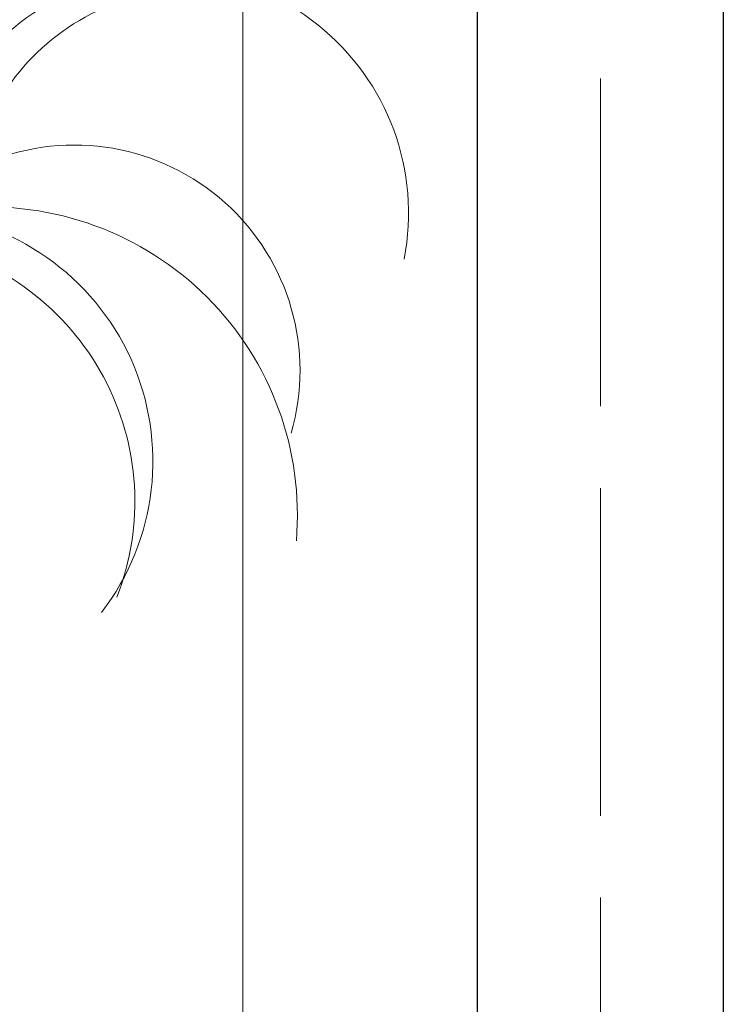
# Model space of a CAD drawing. Units: millimetres. Extents: x 595116 to 630915, y 909473 to 920225.
# Tile 109 of 134: x 629817 to 629843, y 919181 to 919217. Entities that reach past the tile are written whole.
import ezdxf

# ---------------------------------------------------------------- set-up
doc = ezdxf.new("R2010")
doc.units = ezdxf.units.MM
doc.linetypes.add('ACAD_ISO02W100', pattern=[15, 12, -3])
for name, color, linetype, lineweight in [('C-PROP', 7, 'Continuous', 25), ('C-PROP-REF', 240, 'ACAD_ISO02W100', 13), ('L-PLNT', 85, 'Continuous', 13)]:
    doc.layers.add(name, color=color, linetype=linetype, lineweight=lineweight)

# ---------------------------------------------------------------- blocks, each defined once
blk = doc.blocks.new('tree')
for centre, radius, start, end in [((629595.141, 919296.95), 5.184, 352.032, 57.0714), ((629604.232, 919296.737), 3.791, 61.1347, 193.108), ((629569.835, 919289.496), 31.168, 13.149, 20.5076), ((629594.259, 919292.132), 6.965, 7.4001, 94.0059), ((629589.446, 919288.922), 12.167, 24.2477, 54.3726), ((629605.429, 919293.205), 4.185, 348.9977, 176.315), ((629605.915, 919293.144), 3.963, 69.3845, 175.231), ((629595.377, 919292.044), 4.722, 54.2484, 144.2167), ((629594.88, 919291.171), 5.506, 43.8672, 89.4805), ((629597.025, 919289.989), 5.01, 36.0581, 170.6542), ((629603.809, 919290.469), 3.92, 343.886, 112.2662), ((629596.464, 919289.874), 4.4, 52.9074, 159.3471), ((629598.153, 919288.998), 5.103, 105.3576, 208.8973), ((629597.068, 919289.758), 3.768, 80.4816, 161.0664), ((629601.247, 919287.941), 5.545, 101.0419, 191.8692), ((629614.329, 919289.554), 13.748, 164.5925, 192.323), ((629600.849, 919288.894), 4.324, 322.5461, 85.805), ((629602.329, 919287.957), 5.355, 355.2141, 94.8217), ((629602.391, 919286.088), 6.769, 99.681, 184.5451), ((629600.275, 919288.191), 4.585, 338.7925, 77.6921), ((629626.813, 919287.645), 25.579, 169.0753, 185.2889)]:
    blk.add_arc(centre, radius, start, end)

msp = doc.modelspace()

# ---------------------------------------------------------------- linework, layer by layer
at = {"layer": 'C-PROP'}
for p, q in [((629833.541, 919150.928), (629833.541, 919345.928)), ((629842.541, 919345.928), (629842.541, 919141.928))]:
    msp.add_line(p, q, dxfattribs=at)
at = {"layer": 'C-PROP-REF'}
msp.add_line((629838.041, 920084.928), (629838.041, 919141.928), dxfattribs=at)
at = {"layer": 'L-PLNT'}
msp.add_line((629824.951, 919160.917), (629824.951, 919302.009), dxfattribs=at)

# ---------------------------------------------------------------- block references
at = {"layer": 'L-PLNT', "xscale": 2.107689410566463, "yscale": 2.107689410566463, "zscale": 2.107689410566463}
msp.add_blockref('tree', (-697190.499, -1018374.553), dxfattribs=at)

doc.saveas('drawing.dxf')
